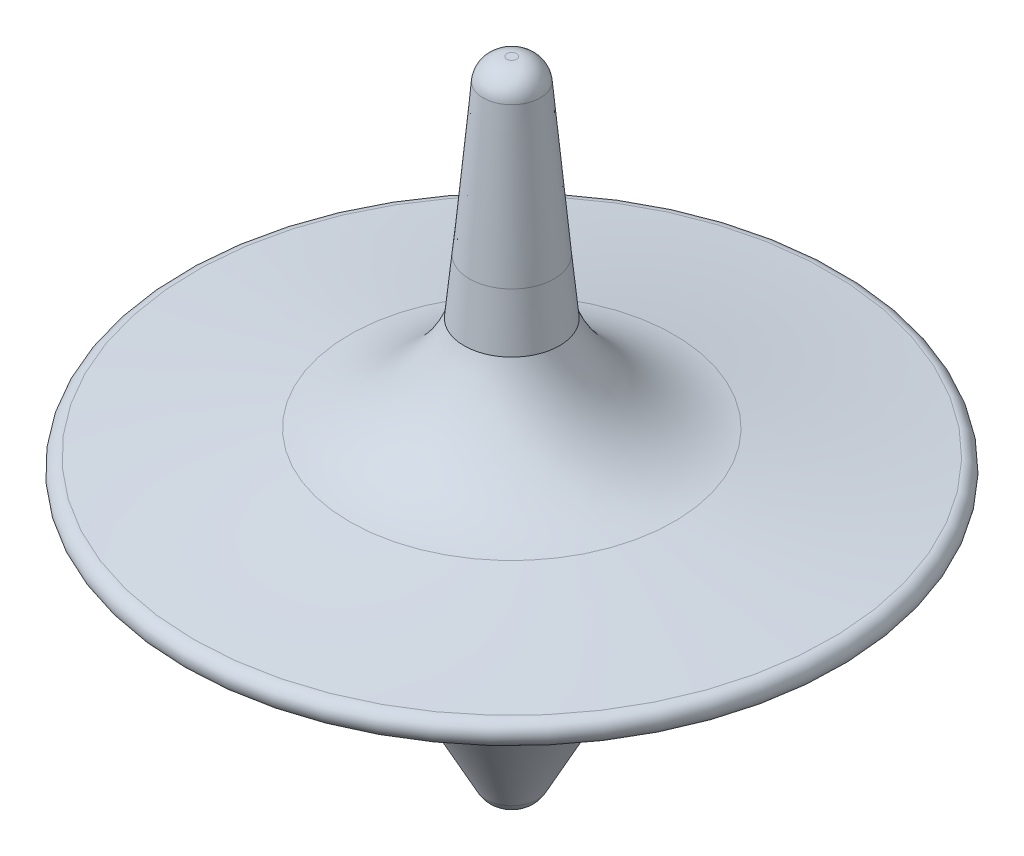
ISO-10303-21;
HEADER;
FILE_DESCRIPTION(('STEP AP214'),'2;1');
FILE_NAME('part.step','',(''),(''),'','','');
FILE_SCHEMA(('AUTOMOTIVE_DESIGN { 1 0 10303 214 1 1 1 1 }'));
ENDSEC;
DATA;
#1=APPLICATION_CONTEXT('core data for automotive mechanical design processes');
#2=APPLICATION_PROTOCOL_DEFINITION('international standard','automotive_design',2000,#1);
#3=PRODUCT_CONTEXT('',#1,'mechanical');
#4=PRODUCT('Part','Part','',(#3));
#5=PRODUCT_RELATED_PRODUCT_CATEGORY('part','',(#4));
#6=PRODUCT_DEFINITION_FORMATION('','',#4);
#7=PRODUCT_DEFINITION_CONTEXT('part definition',#1,'design');
#8=PRODUCT_DEFINITION('design','',#6,#7);
#9=PRODUCT_DEFINITION_SHAPE('','',#8);
#10=(LENGTH_UNIT() NAMED_UNIT(*) SI_UNIT(.MILLI.,.METRE.));
#11=(NAMED_UNIT(*) PLANE_ANGLE_UNIT() SI_UNIT($,.RADIAN.));
#12=(NAMED_UNIT(*) SI_UNIT($,.STERADIAN.) SOLID_ANGLE_UNIT());
#13=UNCERTAINTY_MEASURE_WITH_UNIT(LENGTH_MEASURE(1.E-05),#10,'distance_accuracy_value','');
#14=(GEOMETRIC_REPRESENTATION_CONTEXT(3) GLOBAL_UNCERTAINTY_ASSIGNED_CONTEXT((#13)) GLOBAL_UNIT_ASSIGNED_CONTEXT((#10,
#11,#12)) REPRESENTATION_CONTEXT('',''));
#15=CARTESIAN_POINT('',(0.,0.,0.));
#16=DIRECTION('',(0.,0.,1.));
#17=DIRECTION('',(1.,0.,0.));
#18=AXIS2_PLACEMENT_3D('',#15,#16,#17);
#19=CARTESIAN_POINT('',(0.,-7.49884736579852,0.));
#20=DIRECTION('',(0.,1.,0.));
#21=DIRECTION('',(0.,0.,1.));
#22=AXIS2_PLACEMENT_3D('',#19,#20,#21);
#23=TOROIDAL_SURFACE('',#22,66.6240400436687,2.49999999999997);
#24=CARTESIAN_POINT('',(0.,-9.99828033329375,0.));
#25=DIRECTION('',(0.,1.,0.));
#26=DIRECTION('',(0.,0.,1.));
#27=AXIS2_PLACEMENT_3D('',#24,#25,#26);
#28=CIRCLE('',#27,66.5707968187685);
#29=CARTESIAN_POINT('',(0.,-9.99828033329375,66.5707968187685));
#30=VERTEX_POINT('',#29);
#31=EDGE_CURVE('E77',#30,#30,#28,.T.);
#32=ORIENTED_EDGE('',*,*,#31,.T.);
#33=EDGE_LOOP('',(#32));
#34=FACE_BOUND('',#33,.T.);
#35=CARTESIAN_POINT('',(0.,-5.00000000000017,0.));
#36=DIRECTION('',(0.,1.,0.));
#37=DIRECTION('',(0.,0.,1.));
#38=AXIS2_PLACEMENT_3D('',#35,#36,#37);
#39=CIRCLE('',#38,66.6999468446918);
#40=CARTESIAN_POINT('',(0.,-5.00000000000017,66.6999468446918));
#41=VERTEX_POINT('',#40);
#42=EDGE_CURVE('E10',#41,#41,#39,.T.);
#43=ORIENTED_EDGE('',*,*,#42,.F.);
#44=EDGE_LOOP('',(#43));
#45=FACE_BOUND('',#44,.T.);
#46=ADVANCED_FACE('F39',(#34,#45),#23,.T.);
#47=CARTESIAN_POINT('',(0.,499.397364721149,0.));
#48=DIRECTION('',(0.,1.,0.));
#49=DIRECTION('',(0.,0.,1.));
#50=AXIS2_PLACEMENT_3D('',#47,#48,#49);
#51=DEGENERATE_TOROIDAL_SURFACE('',#50,127.092814489479,508.,.T.);
#52=CARTESIAN_POINT('',(0.,0.,0.));
#53=DIRECTION('',(0.,1.,0.));
#54=DIRECTION('',(0.,0.,1.));
#55=AXIS2_PLACEMENT_3D('',#52,#53,#54);
#56=CIRCLE('',#55,34.);
#57=CARTESIAN_POINT('',(0.,0.,34.));
#58=VERTEX_POINT('',#57);
#59=EDGE_CURVE('E44',#58,#58,#56,.T.);
#60=ORIENTED_EDGE('',*,*,#59,.F.);
#61=EDGE_LOOP('',(#60));
#62=FACE_BOUND('',#61,.T.);
#63=ORIENTED_EDGE('',*,*,#42,.T.);
#64=EDGE_LOOP('',(#63));
#65=FACE_BOUND('',#64,.T.);
#66=ADVANCED_FACE('F106',(#62,#65),#51,.F.);
#67=CARTESIAN_POINT('',(0.,31.458101714718,0.));
#68=DIRECTION('',(0.,1.,0.));
#69=DIRECTION('',(0.,0.,1.));
#70=AXIS2_PLACEMENT_3D('',#67,#68,#69);
#71=TOROIDAL_SURFACE('',#70,39.8641142985499,32.);
#72=CARTESIAN_POINT('',(0.,19.9631168446476,0.));
#73=DIRECTION('',(0.,1.,0.));
#74=DIRECTION('',(0.,0.,1.));
#75=AXIS2_PLACEMENT_3D('',#72,#73,#74);
#76=CIRCLE('',#75,9.99999999999988);
#77=CARTESIAN_POINT('',(0.,19.9631168446476,9.99999999999988));
#78=VERTEX_POINT('',#77);
#79=EDGE_CURVE('E47',#78,#78,#76,.T.);
#80=ORIENTED_EDGE('',*,*,#79,.F.);
#81=EDGE_LOOP('',(#80));
#82=FACE_BOUND('',#81,.T.);
#83=ORIENTED_EDGE('',*,*,#59,.T.);
#84=EDGE_LOOP('',(#83));
#85=FACE_BOUND('',#84,.T.);
#86=ADVANCED_FACE('F109',(#82,#85),#71,.F.);
#87=CARTESIAN_POINT('',(0.,111.483377713465,0.));
#88=DIRECTION('',(0.,1.,0.));
#89=DIRECTION('',(0.,0.,1.));
#90=AXIS2_PLACEMENT_3D('',#87,#88,#89);
#91=TOROIDAL_SURFACE('',#90,885.227994210939,880.);
#92=ORIENTED_EDGE('',*,*,#79,.T.);
#93=EDGE_LOOP('',(#92));
#94=FACE_BOUND('',#93,.T.);
#95=CARTESIAN_POINT('',(0.,31.5328825892603,0.));
#96=DIRECTION('',(0.,1.,0.));
#97=DIRECTION('',(0.,0.,1.));
#98=AXIS2_PLACEMENT_3D('',#95,#96,#97);
#99=CIRCLE('',#98,8.86738445637268);
#100=CARTESIAN_POINT('',(0.,31.5328825892603,8.86738445637268));
#101=VERTEX_POINT('',#100);
#102=EDGE_CURVE('E52',#101,#101,#99,.T.);
#103=ORIENTED_EDGE('',*,*,#102,.F.);
#104=EDGE_LOOP('',(#103));
#105=FACE_BOUND('',#104,.T.);
#106=ADVANCED_FACE('F113',(#94,#105),#91,.F.);
#107=CARTESIAN_POINT('',(0.,62.9631168446475,0.));
#108=DIRECTION('',(0.,-1.,0.));
#109=DIRECTION('',(0.,0.,-1.));
#110=AXIS2_PLACEMENT_3D('',#107,#108,#109);
#111=CONICAL_SURFACE('',#110,5.99999999999996,0.0909782887305641);
#112=ORIENTED_EDGE('',*,*,#102,.T.);
#113=EDGE_LOOP('',(#112));
#114=FACE_BOUND('',#113,.T.);
#115=CARTESIAN_POINT('',(0.,62.9631168446475,0.));
#116=DIRECTION('',(0.,1.,0.));
#117=DIRECTION('',(0.,0.,1.));
#118=AXIS2_PLACEMENT_3D('',#115,#116,#117);
#119=CIRCLE('',#118,5.99999999999996);
#120=CARTESIAN_POINT('',(0.,62.9631168446475,5.99999999999996));
#121=VERTEX_POINT('',#120);
#122=EDGE_CURVE('E59',#121,#121,#119,.T.);
#123=ORIENTED_EDGE('',*,*,#122,.F.);
#124=EDGE_LOOP('',(#123));
#125=FACE_BOUND('',#124,.T.);
#126=ADVANCED_FACE('F121',(#114,#125),#111,.T.);
#127=CARTESIAN_POINT('',(0.,62.5,0.));
#128=DIRECTION('',(0.,1.,0.));
#129=DIRECTION('',(0.,0.,1.));
#130=AXIS2_PLACEMENT_3D('',#127,#128,#129);
#131=DEGENERATE_TOROIDAL_SURFACE('',#130,1.02149392003945,5.,.T.);
#132=CARTESIAN_POINT('',(0.,67.5,0.));
#133=DIRECTION('',(0.,1.,0.));
#134=DIRECTION('',(0.,0.,1.));
#135=AXIS2_PLACEMENT_3D('',#132,#133,#134);
#136=CIRCLE('',#135,1.02149392003945);
#137=CARTESIAN_POINT('',(0.,67.5,1.02149392003945));
#138=VERTEX_POINT('',#137);
#139=EDGE_CURVE('E62',#138,#138,#136,.T.);
#140=ORIENTED_EDGE('',*,*,#139,.F.);
#141=EDGE_LOOP('',(#140));
#142=FACE_BOUND('',#141,.T.);
#143=ORIENTED_EDGE('',*,*,#122,.T.);
#144=EDGE_LOOP('',(#143));
#145=FACE_BOUND('',#144,.T.);
#146=ADVANCED_FACE('F125',(#142,#145),#131,.T.);
#147=CARTESIAN_POINT('',(0.,67.5,0.));
#148=DIRECTION('',(0.,1.,0.));
#149=DIRECTION('',(0.,0.,1.));
#150=AXIS2_PLACEMENT_3D('',#147,#148,#149);
#151=PLANE('',#150);
#152=ORIENTED_EDGE('',*,*,#139,.T.);
#153=EDGE_LOOP('',(#152));
#154=FACE_BOUND('',#153,.T.);
#155=ADVANCED_FACE('F129',(#154),#151,.T.);
#156=CARTESIAN_POINT('',(1.00535316910453E-12,-67.5,0.));
#157=DIRECTION('',(0.,1.,0.));
#158=DIRECTION('',(0.,0.,1.));
#159=AXIS2_PLACEMENT_3D('',#156,#157,#158);
#160=PLANE('',#159);
#161=CARTESIAN_POINT('',(0.,-67.5,0.));
#162=DIRECTION('',(0.,1.,0.));
#163=DIRECTION('',(0.,0.,1.));
#164=AXIS2_PLACEMENT_3D('',#161,#162,#163);
#165=CIRCLE('',#164,0.931762793230006);
#166=CARTESIAN_POINT('',(0.,-67.5,0.931762793230006));
#167=VERTEX_POINT('',#166);
#168=EDGE_CURVE('E61',#167,#167,#165,.T.);
#169=ORIENTED_EDGE('',*,*,#168,.F.);
#170=EDGE_LOOP('',(#169));
#171=FACE_BOUND('',#170,.T.);
#172=ADVANCED_FACE('F105',(#171),#160,.F.);
#173=CARTESIAN_POINT('',(0.,-62.5,0.));
#174=DIRECTION('',(0.,1.,0.));
#175=DIRECTION('',(0.,0.,1.));
#176=AXIS2_PLACEMENT_3D('',#173,#174,#175);
#177=DEGENERATE_TOROIDAL_SURFACE('',#176,0.931762793230005,4.99999999999999,.T.);
#178=ORIENTED_EDGE('',*,*,#168,.T.);
#179=EDGE_LOOP('',(#178));
#180=FACE_BOUND('',#179,.T.);
#181=CARTESIAN_POINT('',(0.,-64.7438485385685,0.));
#182=DIRECTION('',(0.,1.,0.));
#183=DIRECTION('',(0.,0.,1.));
#184=AXIS2_PLACEMENT_3D('',#181,#182,#183);
#185=CIRCLE('',#184,5.40000000000002);
#186=CARTESIAN_POINT('',(0.,-64.7438485385685,5.40000000000002));
#187=VERTEX_POINT('',#186);
#188=EDGE_CURVE('E67',#187,#187,#185,.T.);
#189=ORIENTED_EDGE('',*,*,#188,.F.);
#190=EDGE_LOOP('',(#189));
#191=FACE_BOUND('',#190,.T.);
#192=ADVANCED_FACE('F96',(#180,#191),#177,.T.);
#193=CARTESIAN_POINT('',(0.,-208.350155006952,0.));
#194=DIRECTION('',(0.,1.,0.));
#195=DIRECTION('',(0.,0.,1.));
#196=AXIS2_PLACEMENT_3D('',#193,#194,#195);
#197=DEGENERATE_TOROIDAL_SURFACE('',#196,291.367181233282,320.,.T.);
#198=ORIENTED_EDGE('',*,*,#188,.T.);
#199=EDGE_LOOP('',(#198));
#200=FACE_BOUND('',#199,.T.);
#201=CARTESIAN_POINT('',(0.,-23.5166494436719,0.));
#202=DIRECTION('',(0.,1.,0.));
#203=DIRECTION('',(0.,0.,1.));
#204=AXIS2_PLACEMENT_3D('',#201,#202,#203);
#205=CIRCLE('',#204,30.1458665953128);
#206=CARTESIAN_POINT('',(0.,-23.5166494436719,30.1458665953128));
#207=VERTEX_POINT('',#206);
#208=EDGE_CURVE('E70',#207,#207,#205,.T.);
#209=ORIENTED_EDGE('',*,*,#208,.F.);
#210=EDGE_LOOP('',(#209));
#211=FACE_BOUND('',#210,.T.);
#212=ADVANCED_FACE('F93',(#200,#211),#197,.F.);
#213=CARTESIAN_POINT('',(0.,-42.,0.));
#214=DIRECTION('',(0.,1.,0.));
#215=DIRECTION('',(0.,0.,1.));
#216=AXIS2_PLACEMENT_3D('',#213,#214,#215);
#217=TOROIDAL_SURFACE('',#216,56.2679980591097,32.);
#218=CARTESIAN_POINT('',(0.,-9.99999999999995,0.));
#219=DIRECTION('',(0.,1.,0.));
#220=DIRECTION('',(0.,0.,1.));
#221=AXIS2_PLACEMENT_3D('',#218,#219,#220);
#222=CIRCLE('',#221,56.2679980591097);
#223=CARTESIAN_POINT('',(0.,-9.99999999999995,56.2679980591097));
#224=VERTEX_POINT('',#223);
#225=EDGE_CURVE('E71',#224,#224,#222,.T.);
#226=ORIENTED_EDGE('',*,*,#225,.F.);
#227=EDGE_LOOP('',(#226));
#228=FACE_BOUND('',#227,.T.);
#229=ORIENTED_EDGE('',*,*,#208,.T.);
#230=EDGE_LOOP('',(#229));
#231=FACE_BOUND('',#230,.T.);
#232=ADVANCED_FACE('F85',(#228,#231),#217,.F.);
#233=CARTESIAN_POINT('',(0.,-249.94384521284,0.));
#234=DIRECTION('',(0.,1.,0.));
#235=DIRECTION('',(0.,0.,1.));
#236=AXIS2_PLACEMENT_3D('',#233,#234,#235);
#237=DEGENERATE_TOROIDAL_SURFACE('',#236,61.4594472283437,240.,.T.);
#238=ORIENTED_EDGE('',*,*,#31,.F.);
#239=EDGE_LOOP('',(#238));
#240=FACE_BOUND('',#239,.T.);
#241=ORIENTED_EDGE('',*,*,#225,.T.);
#242=EDGE_LOOP('',(#241));
#243=FACE_BOUND('',#242,.T.);
#244=ADVANCED_FACE('F82',(#240,#243),#237,.F.);
#245=CLOSED_SHELL('',(#46,#66,#86,#106,#126,#146,#155,#172,#192,#212,#232,#244));
#246=MANIFOLD_SOLID_BREP('B2',#245);
#247=ADVANCED_BREP_SHAPE_REPRESENTATION('',(#18,#246),#14);
#248=SHAPE_DEFINITION_REPRESENTATION(#9,#247);
ENDSEC;
END-ISO-10303-21;
